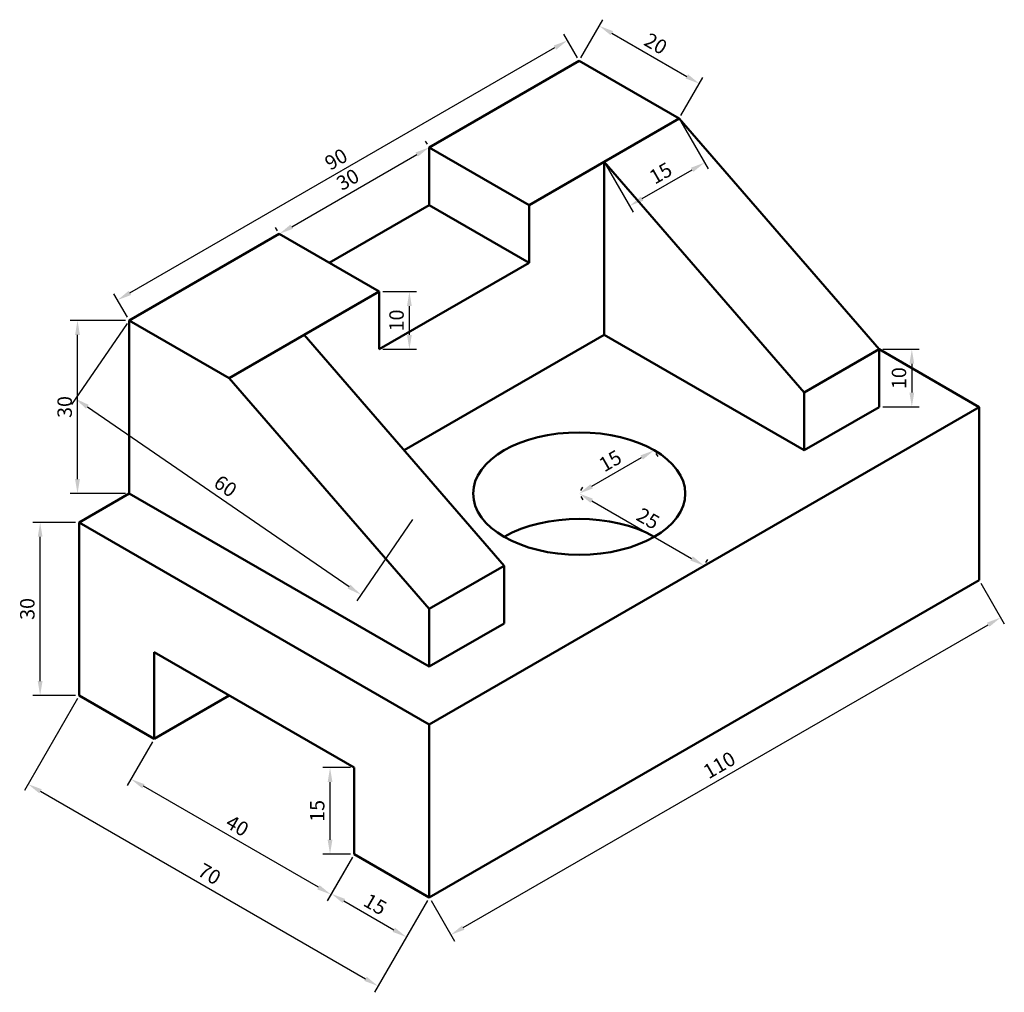
# Model space of a CAD drawing. Units: millimetres. Extents: x 2421 to 2592, y 893 to 1062.
import ezdxf

# ---------------------------------------------------------------- set-up
doc = ezdxf.new("R2010")
doc.units = ezdxf.units.MM
doc.layers.add('M-DIMS', color=2, linetype='Continuous', lineweight=25)
doc.layers.add('M-OUTL', color=7, linetype='Continuous', lineweight=50)
doc.styles.get("Standard").update_dxf_attribs({"font": 'arial.ttf'})
doc.dimstyles.new('ISO-25', dxfattribs={"dimtxt": 2.5, "dimasz": 2.5, "dimexe": 1.25, "dimexo": 0.625, "dimtad": 1, "dimtxsty": 'Standard', "dimcen": 2.5, "dimadec": 0, "dimazin": 0, "dimtfac": 1, "dimtmove": 0, "dimatfit": 3, "dimfxl": 1, "dimarcsym": 0})

# ---------------------------------------------------------------- blocks, each defined once
blk = doc.blocks.new('*D1')
at = {"layer": 'Defpoints', "color": 0, "transparency": 16777216}
for p in [(2424.82, 974.94), (2431.59, 974.94), (2431.59, 944.94)]:
    blk.add_point(p, dxfattribs=at)
at = {"layer": 'M-DIMS', "color": 0, "lineweight": -2, "transparency": 16777216}
for p, q in [((2430.97, 974.94), (2423.57, 974.94)), ((2424.82, 947.44), (2424.82, 972.44)), ((2430.97, 944.94), (2423.57, 944.94))]:
    blk.add_line(p, q, dxfattribs=at)
at = {"layer": 'M-DIMS', "color": 0, "transparency": 16777216}
for points in [[(2424.4, 972.44), (2425.23, 972.44), (2424.82, 974.94)], [(2424.4, 947.44), (2425.23, 947.44), (2424.82, 944.94)]]:
    blk.add_solid(points, dxfattribs=at)
at = {"layer": 'M-DIMS', "color": 0, "transparency": 16777216, "insert": (2422.92, 959.94), "char_height": 2.5, "attachment_point": 5, "rotation": 90}
blk.add_mtext('30', dxfattribs=at)
blk = doc.blocks.new('*D2')
at = {"layer": 'Defpoints', "color": 0, "transparency": 16777216}
for p in [(2431.29, 1009.94), (2440.25, 1009.94), (2440.25, 979.94)]:
    blk.add_point(p, dxfattribs=at)
at = {"layer": 'M-DIMS', "color": 0, "lineweight": -2, "transparency": 16777216}
for p, q in [((2439.63, 1009.94), (2430.04, 1009.94)), ((2431.29, 982.44), (2431.29, 1007.44)), ((2439.63, 979.94), (2430.04, 979.94))]:
    blk.add_line(p, q, dxfattribs=at)
at = {"layer": 'M-DIMS', "color": 0, "transparency": 16777216}
for points in [[(2430.87, 1007.44), (2431.71, 1007.44), (2431.29, 1009.94)], [(2430.87, 982.44), (2431.71, 982.44), (2431.29, 979.94)]]:
    blk.add_solid(points, dxfattribs=at)
at = {"layer": 'M-DIMS', "color": 0, "transparency": 16777216, "insert": (2429.39, 994.94), "char_height": 2.5, "attachment_point": 5, "rotation": 90}
blk.add_mtext('30', dxfattribs=at)
blk = doc.blocks.new('*D3')
at = {"layer": 'Defpoints', "color": 0, "transparency": 16777216}
for p in [(2440.25, 1009.94), (2489.7, 975.96), (2480.39, 962.4)]:
    blk.add_point(p, dxfattribs=at)
at = {"layer": 'M-DIMS', "color": 0, "lineweight": -2, "transparency": 16777216}
for p, q in [((2439.9, 1009.42), (2430.23, 995.35)), ((2433, 994.96), (2478.33, 963.81)), ((2489.35, 975.44), (2479.68, 961.37))]:
    blk.add_line(p, q, dxfattribs=at)
at = {"layer": 'M-DIMS', "color": 0, "transparency": 16777216}
for points in [[(2433.23, 995.31), (2432.76, 994.62), (2430.94, 996.38)], [(2478.56, 964.16), (2478.09, 963.47), (2480.39, 962.4)]]:
    blk.add_solid(points, dxfattribs=at)
at = {"layer": 'M-DIMS', "color": 0, "transparency": 16777216, "insert": (2456.74, 980.96), "char_height": 2.5, "attachment_point": 5, "rotation": 325.5033}
blk.add_mtext('60', dxfattribs=at)
blk = doc.blocks.new('*D4')
at = {"layer": 'Defpoints', "color": 0, "transparency": 16777216}
for p in [(2516.16, 1058.47), (2518.2, 1054.94), (2440.25, 1009.94)]:
    blk.add_point(p, dxfattribs=at)
at = {"layer": 'M-DIMS', "color": 0, "lineweight": -2, "transparency": 16777216}
for p, q in [((2517.88, 1055.48), (2515.54, 1059.55)), ((2440.38, 1014.72), (2514, 1057.22)), ((2439.94, 1010.48), (2437.59, 1014.55))]:
    blk.add_line(p, q, dxfattribs=at)
at = {"layer": 'M-DIMS', "color": 0, "transparency": 16777216}
for points in [[(2513.79, 1057.58), (2514.2, 1056.85), (2516.16, 1058.47)], [(2440.17, 1015.08), (2440.59, 1014.35), (2438.22, 1013.47)]]:
    blk.add_solid(points, dxfattribs=at)
at = {"layer": 'M-DIMS', "color": 0, "transparency": 16777216, "insert": (2476.24, 1037.61), "char_height": 2.5, "attachment_point": 5, "rotation": 30}
blk.add_mtext('90', dxfattribs=at)
blk = doc.blocks.new('*D5')
at = {"layer": 'Defpoints', "color": 0, "transparency": 16777216}
for p in [(2518.2, 1054.94), (2539.01, 1050.98), (2535.52, 1044.94)]:
    blk.add_point(p, dxfattribs=at)
at = {"layer": 'M-DIMS', "color": 0, "lineweight": -2, "transparency": 16777216}
for p, q in [((2518.51, 1055.48), (2522.31, 1062.06)), ((2523.85, 1059.73), (2536.84, 1052.23)), ((2535.83, 1045.48), (2539.63, 1052.06))]:
    blk.add_line(p, q, dxfattribs=at)
at = {"layer": 'M-DIMS', "color": 0, "transparency": 16777216}
for points in [[(2524.06, 1060.09), (2523.64, 1059.37), (2521.69, 1060.98)], [(2537.05, 1052.59), (2536.63, 1051.87), (2539.01, 1050.98)]]:
    blk.add_solid(points, dxfattribs=at)
at = {"layer": 'M-DIMS', "color": 0, "transparency": 16777216, "insert": (2531.3, 1057.63), "char_height": 2.5, "attachment_point": 5, "rotation": 330}
blk.add_mtext('20', dxfattribs=at)
blk = doc.blocks.new('*D6')
at = {"layer": 'Defpoints', "color": 0, "transparency": 16777216}
for p in [(2535.52, 1044.94), (2522.53, 1037.44), (2539.93, 1037.3)]:
    blk.add_point(p, dxfattribs=at)
at = {"layer": 'M-DIMS', "color": 0, "lineweight": -2, "transparency": 16777216}
for p, q in [((2535.83, 1044.4), (2540.55, 1036.21)), ((2522.84, 1036.9), (2527.56, 1028.71)), ((2529.1, 1031.05), (2537.76, 1036.05))]:
    blk.add_line(p, q, dxfattribs=at)
at = {"layer": 'M-DIMS', "color": 0, "transparency": 16777216}
for points in [[(2537.56, 1036.41), (2537.97, 1035.69), (2539.93, 1037.3)], [(2528.9, 1031.41), (2529.31, 1030.69), (2526.94, 1029.8)]]:
    blk.add_solid(points, dxfattribs=at)
at = {"layer": 'M-DIMS', "color": 0, "transparency": 16777216, "insert": (2532.48, 1035.19), "char_height": 2.5, "attachment_point": 5, "rotation": 30}
blk.add_mtext('15', dxfattribs=at)
blk = doc.blocks.new('*D7')
at = {"layer": 'Defpoints', "color": 0, "transparency": 16777216}
for p in [(2518.2, 979.94), (2539.85, 967.44), (2539.85, 967.44)]:
    blk.add_point(p, dxfattribs=at)
at = {"layer": 'M-DIMS', "color": 0, "lineweight": -2, "transparency": 16777216}
for p, q in [((2518.51, 980.48), (2518.82, 981.02)), ((2520.36, 978.69), (2537.68, 968.69)), ((2540.16, 967.98), (2540.47, 968.52))]:
    blk.add_line(p, q, dxfattribs=at)
at = {"layer": 'M-DIMS', "color": 0, "transparency": 16777216}
for points in [[(2520.57, 979.05), (2520.15, 978.33), (2518.2, 979.94)], [(2537.89, 969.05), (2537.47, 968.33), (2539.85, 967.44)]]:
    blk.add_solid(points, dxfattribs=at)
at = {"layer": 'M-DIMS', "color": 0, "transparency": 16777216, "insert": (2529.97, 975.33), "char_height": 2.5, "attachment_point": 5, "rotation": 330}
blk.add_mtext('25', dxfattribs=at)
blk = doc.blocks.new('*D8')
at = {"layer": 'Defpoints', "color": 0, "transparency": 16777216}
for p in [(2531.19, 987.44), (2531.19, 987.44), (2518.2, 979.94)]:
    blk.add_point(p, dxfattribs=at)
at = {"layer": 'M-DIMS', "color": 0, "lineweight": -2, "transparency": 16777216}
for p, q in [((2520.36, 981.19), (2529.02, 986.19)), ((2531.5, 986.9), (2531.81, 986.36)), ((2518.51, 979.4), (2518.82, 978.86))]:
    blk.add_line(p, q, dxfattribs=at)
at = {"layer": 'M-DIMS', "color": 0, "transparency": 16777216}
for points in [[(2528.81, 986.55), (2529.23, 985.83), (2531.19, 987.44)], [(2520.15, 981.55), (2520.57, 980.83), (2518.2, 979.94)]]:
    blk.add_solid(points, dxfattribs=at)
at = {"layer": 'M-DIMS', "color": 0, "transparency": 16777216, "insert": (2523.74, 985.33), "char_height": 2.5, "attachment_point": 5, "rotation": 30}
blk.add_mtext('15', dxfattribs=at)
blk = doc.blocks.new('*D9')
at = {"layer": 'Defpoints', "color": 0, "transparency": 16777216}
for p in [(2570.16, 1004.94), (2570.16, 994.94), (2575.82, 994.94)]:
    blk.add_point(p, dxfattribs=at)
at = {"layer": 'M-DIMS', "color": 0, "lineweight": -2, "transparency": 16777216}
for p, q in [((2570.78, 1004.94), (2577.07, 1004.94)), ((2575.82, 1002.44), (2575.82, 997.44)), ((2570.78, 994.94), (2577.07, 994.94))]:
    blk.add_line(p, q, dxfattribs=at)
at = {"layer": 'M-DIMS', "color": 0, "transparency": 16777216}
for points in [[(2575.41, 1002.44), (2576.24, 1002.44), (2575.82, 1004.94)], [(2575.41, 997.44), (2576.24, 997.44), (2575.82, 994.94)]]:
    blk.add_solid(points, dxfattribs=at)
at = {"layer": 'M-DIMS', "color": 0, "transparency": 16777216, "insert": (2573.92, 999.94), "char_height": 2.5, "attachment_point": 5, "rotation": 90}
blk.add_mtext('10', dxfattribs=at)
blk = doc.blocks.new('*D10')
at = {"layer": 'Defpoints', "color": 0, "transparency": 16777216}
for p in [(2483.56, 1014.94), (2488.78, 1014.94), (2483.56, 1004.94)]:
    blk.add_point(p, dxfattribs=at)
at = {"layer": 'M-DIMS', "color": 0, "lineweight": -2, "transparency": 16777216}
for p, q in [((2484.18, 1014.94), (2490.03, 1014.94)), ((2488.78, 1007.44), (2488.78, 1012.44)), ((2484.18, 1004.94), (2490.03, 1004.94))]:
    blk.add_line(p, q, dxfattribs=at)
at = {"layer": 'M-DIMS', "color": 0, "transparency": 16777216}
for points in [[(2488.37, 1012.44), (2489.2, 1012.44), (2488.78, 1014.94)], [(2488.37, 1007.44), (2489.2, 1007.44), (2488.78, 1004.94)]]:
    blk.add_solid(points, dxfattribs=at)
at = {"layer": 'M-DIMS', "color": 0, "transparency": 16777216, "insert": (2486.88, 1009.94), "char_height": 2.5, "attachment_point": 5, "rotation": 90}
blk.add_mtext('10', dxfattribs=at)
blk = doc.blocks.new('*D11')
at = {"layer": 'Defpoints', "color": 0, "transparency": 16777216}
for p in [(2475.04, 932.44), (2479.23, 932.44), (2479.23, 917.44)]:
    blk.add_point(p, dxfattribs=at)
at = {"layer": 'M-DIMS', "color": 0, "lineweight": -2, "transparency": 16777216}
for p, q in [((2478.6, 932.44), (2473.79, 932.44)), ((2475.04, 919.94), (2475.04, 929.94)), ((2478.6, 917.44), (2473.79, 917.44))]:
    blk.add_line(p, q, dxfattribs=at)
at = {"layer": 'M-DIMS', "color": 0, "transparency": 16777216}
for points in [[(2474.62, 929.94), (2475.45, 929.94), (2475.04, 932.44)], [(2474.62, 919.94), (2475.45, 919.94), (2475.04, 917.44)]]:
    blk.add_solid(points, dxfattribs=at)
at = {"layer": 'M-DIMS', "color": 0, "transparency": 16777216, "insert": (2473.14, 924.94), "char_height": 2.5, "attachment_point": 5, "rotation": 90}
blk.add_mtext('15', dxfattribs=at)
blk = doc.blocks.new('*D12')
at = {"layer": 'Defpoints', "color": 0, "transparency": 16777216}
for p in [(2587.48, 964.94), (2591.22, 958.46), (2492.22, 909.94)]:
    blk.add_point(p, dxfattribs=at)
at = {"layer": 'M-DIMS', "color": 0, "lineweight": -2, "transparency": 16777216}
for p, q in [((2587.79, 964.4), (2591.84, 957.38)), ((2498.12, 904.71), (2589.05, 957.21)), ((2492.53, 909.4), (2496.58, 902.38))]:
    blk.add_line(p, q, dxfattribs=at)
at = {"layer": 'M-DIMS', "color": 0, "transparency": 16777216}
for points in [[(2588.84, 957.57), (2589.26, 956.85), (2591.22, 958.46)], [(2497.91, 905.07), (2498.33, 904.35), (2495.95, 903.46)]]:
    blk.add_solid(points, dxfattribs=at)
at = {"layer": 'M-DIMS', "color": 0, "transparency": 16777216, "insert": (2542.63, 932.61), "char_height": 2.5, "attachment_point": 5, "rotation": 30}
blk.add_mtext('110', dxfattribs=at)
blk = doc.blocks.new('*D13')
at = {"layer": 'Defpoints', "color": 0, "transparency": 16777216}
for p in [(2444.58, 937.44), (2440.55, 930.45), (2479.23, 917.44)]:
    blk.add_point(p, dxfattribs=at)
at = {"layer": 'M-DIMS', "color": 0, "lineweight": -2, "transparency": 16777216}
for p, q in [((2444.27, 936.9), (2439.92, 929.36)), ((2473.02, 911.7), (2442.71, 929.2)), ((2478.91, 916.9), (2474.56, 909.36))]:
    blk.add_line(p, q, dxfattribs=at)
at = {"layer": 'M-DIMS', "color": 0, "transparency": 16777216}
for points in [[(2442.92, 929.56), (2442.51, 928.84), (2440.55, 930.45)], [(2473.23, 912.06), (2472.82, 911.34), (2475.19, 910.45)]]:
    blk.add_solid(points, dxfattribs=at)
at = {"layer": 'M-DIMS', "color": 0, "transparency": 16777216, "insert": (2458.82, 922.09), "char_height": 2.5, "attachment_point": 5, "rotation": 330}
blk.add_mtext('40', dxfattribs=at)
blk = doc.blocks.new('*D14')
at = {"layer": 'Defpoints', "color": 0, "transparency": 16777216}
for p in [(2431.59, 944.94), (2492.22, 909.94), (2483.35, 894.58)]:
    blk.add_point(p, dxfattribs=at)
at = {"layer": 'M-DIMS', "color": 0, "lineweight": -2, "transparency": 16777216}
for p, q in [((2431.28, 944.4), (2422.1, 928.5)), ((2424.89, 928.33), (2481.18, 895.83)), ((2491.9, 909.4), (2482.72, 893.5))]:
    blk.add_line(p, q, dxfattribs=at)
at = {"layer": 'M-DIMS', "color": 0, "transparency": 16777216}
for points in [[(2425.1, 928.69), (2424.68, 927.97), (2422.73, 929.58)], [(2481.39, 896.19), (2480.98, 895.47), (2483.35, 894.58)]]:
    blk.add_solid(points, dxfattribs=at)
at = {"layer": 'M-DIMS', "color": 0, "transparency": 16777216, "insert": (2453.99, 913.73), "char_height": 2.5, "attachment_point": 5, "rotation": 330}
blk.add_mtext('70', dxfattribs=at)
blk = doc.blocks.new('*D15')
at = {"layer": 'Defpoints', "color": 0, "transparency": 16777216}
for p in [(2479.23, 917.44), (2492.22, 909.94), (2488.26, 903.08)]:
    blk.add_point(p, dxfattribs=at)
at = {"layer": 'M-DIMS', "color": 0, "lineweight": -2, "transparency": 16777216}
for p, q in [((2478.91, 916.9), (2474.64, 909.5)), ((2477.43, 909.33), (2486.09, 904.33)), ((2491.9, 909.4), (2487.63, 902))]:
    blk.add_line(p, q, dxfattribs=at)
at = {"layer": 'M-DIMS', "color": 0, "transparency": 16777216}
for points in [[(2477.64, 909.69), (2477.22, 908.97), (2475.27, 910.58)], [(2486.3, 904.69), (2485.88, 903.97), (2488.26, 903.08)]]:
    blk.add_solid(points, dxfattribs=at)
at = {"layer": 'M-DIMS', "color": 0, "transparency": 16777216, "insert": (2482.71, 908.48), "char_height": 2.5, "attachment_point": 5, "rotation": 330}
blk.add_mtext('15', dxfattribs=at)
blk = doc.blocks.new('*D16')
at = {"layer": 'Defpoints', "color": 0, "transparency": 16777216}
for p in [(2492.22, 1039.94), (2492.22, 1039.94), (2466.24, 1024.94)]:
    blk.add_point(p, dxfattribs=at)
at = {"layer": 'M-DIMS', "color": 0, "lineweight": -2, "transparency": 16777216}
for p, q in [((2491.9, 1040.48), (2491.59, 1041.02)), ((2468.4, 1026.19), (2490.05, 1038.69)), ((2465.92, 1025.48), (2465.61, 1026.02))]:
    blk.add_line(p, q, dxfattribs=at)
at = {"layer": 'M-DIMS', "color": 0, "transparency": 16777216}
for points in [[(2489.84, 1039.05), (2490.26, 1038.33), (2492.22, 1039.94)], [(2468.19, 1026.55), (2468.61, 1025.83), (2466.24, 1024.94)]]:
    blk.add_solid(points, dxfattribs=at)
at = {"layer": 'M-DIMS', "color": 0, "transparency": 16777216, "insert": (2478.27, 1034.09), "char_height": 2.5, "attachment_point": 5, "rotation": 30}
blk.add_mtext('30', dxfattribs=at)

msp = doc.modelspace()

# ---------------------------------------------------------------- linework, layer by layer
at = {"layer": 'M-OUTL'}
for p, q in [((2492.216, 1039.938), (2518.197, 1054.938)), ((2518.197, 1054.938), (2535.517, 1044.938)), ((2535.517, 1044.938), (2509.536, 1029.938)), ((2535.517, 1044.938), (2570.158, 1004.938)), ((2509.536, 1029.938), (2492.216, 1039.938)), ((2492.216, 1029.938), (2492.216, 1039.938)), ((2522.527, 1007.438), (2522.527, 1037.438)), ((2522.527, 1037.438), (2557.168, 997.438)), ((2492.216, 1029.938), (2474.895, 1019.938)), ((2509.536, 1019.938), (2492.216, 1029.938)), ((2509.536, 1019.938), (2509.536, 1029.938)), ((2440.254, 1009.938), (2466.235, 1024.938)), ((2466.235, 1024.938), (2483.556, 1014.938)), ((2483.556, 1004.938), (2509.536, 1019.938)), ((2457.575, 999.938), (2483.556, 1014.938)), ((2483.556, 1014.938), (2483.556, 1004.938)), ((2440.254, 979.938), (2440.254, 1009.938)), ((2440.254, 1009.938), (2457.575, 999.938)), ((2470.565, 1007.438), (2505.206, 967.438)), ((2522.527, 1007.438), (2487.886, 987.438)), ((2557.168, 987.438), (2522.527, 1007.438)), ((2570.158, 1004.938), (2557.168, 997.438)), ((2570.158, 994.938), (2570.158, 1004.938)), ((2578.818, 999.938), (2570.158, 1004.938)), ((2457.575, 999.938), (2492.216, 959.938)), ((2587.479, 994.938), (2578.818, 999.938)), ((2557.168, 997.438), (2557.168, 987.438)), ((2587.479, 994.938), (2492.216, 939.938)), ((2557.168, 987.438), (2570.158, 994.938)), ((2587.479, 964.938), (2587.479, 994.938)), ((2431.594, 974.938), (2440.254, 979.938)), ((2440.254, 979.938), (2492.216, 949.938)), ((2431.594, 944.938), (2431.594, 974.938)), ((2431.594, 974.938), (2492.216, 939.938)), ((2505.206, 967.438), (2492.216, 959.938)), ((2505.206, 957.438), (2505.206, 967.438)), ((2492.216, 909.938), (2587.479, 964.938)), ((2492.216, 959.938), (2492.216, 949.938)), ((2492.216, 949.938), (2505.206, 957.438)), ((2479.225, 932.438), (2444.584, 952.438)), ((2444.584, 952.438), (2444.584, 937.438)), ((2444.584, 937.438), (2431.594, 944.938)), ((2444.584, 937.438), (2457.575, 944.938)), ((2492.216, 939.938), (2492.216, 909.938)), ((2479.225, 917.438), (2479.225, 932.438)), ((2492.216, 909.938), (2479.225, 917.438))]:
    msp.add_line(p, q, dxfattribs=at)
msp.add_ellipse((2518.197, 979.938), major_axis=(-18.371, 0), ratio=0.5773503, dxfattribs=at)
msp.add_ellipse((2518.197, 964.938), major_axis=(18.371, 0), ratio=0.5773503, start_param=0.7853982, end_param=2.3561945, dxfattribs=at)

# ---------------------------------------------------------------- dimensions: what is measured, and where the dimension line sits
at = {"layer": 'M-DIMS'}
for p1, p2, distance, picture, middle in [((2518.197, 1054.938), (2535.517, 1044.938), 6.979, '*D5', (2531.297, 1057.629)), ((2440.254, 1009.938), (2518.197, 1054.938), 4.073, '*D4', (2476.238, 1037.612)), ((2522.527, 1037.438), (2535.517, 1044.938), -8.824, '*D6', (2532.483, 1035.193)), ((2466.235, 1024.938), (2492.216, 1039.938), 0, '*D16', (2478.274, 1034.085)), ((2440.254, 1009.938), (2489.704, 975.956), -16.45, '*D3', (2456.739, 980.957)), ((2518.197, 979.938), (2531.187, 987.438), 0, '*D8', (2523.741, 985.335)), ((2518.197, 979.938), (2539.847, 967.438), 0, '*D7', (2529.973, 975.335)), ((2492.216, 909.938), (2587.479, 964.938), -7.477, '*D12', (2542.635, 932.61)), ((2431.594, 944.938), (2492.216, 909.938), -17.735, '*D14', (2453.988, 913.726)), ((2479.225, 917.438), (2444.584, 937.438), 8.072, '*D13', (2458.82, 922.094)), ((2479.225, 917.438), (2492.216, 909.938), -7.917, '*D15', (2482.713, 908.478))]:
    dim = msp.add_aligned_dim(p1=p1, p2=p2, distance=distance, dimstyle='ISO-25', override={"dimclrd": 0, "dimclre": 0, "dimclrt": 0}, dxfattribs=at)
    dim.commit()
    dim.dimension.update_dxf_attribs({"geometry": picture, "text_midpoint": middle})
for base, p1, p2, picture, middle in [((2488.785, 1014.938), (2483.556, 1004.938), (2483.556, 1014.938), '*D10', (2486.883, 1009.938)), ((2431.291, 1009.938), (2440.254, 979.938), (2440.254, 1009.938), '*D2', (2429.389, 994.938)), ((2575.822, 994.938), (2570.158, 1004.938), (2570.158, 994.938), '*D9', (2573.921, 999.938)), ((2424.818, 974.938), (2431.594, 944.938), (2431.594, 974.938), '*D1', (2422.916, 959.938)), ((2475.037, 932.438), (2479.225, 917.438), (2479.225, 932.438), '*D11', (2473.135, 924.938))]:
    dim = msp.add_linear_dim(base=base, p1=p1, p2=p2, angle=90, dimstyle='ISO-25', override={"dimclrd": 0, "dimclre": 0, "dimclrt": 0}, dxfattribs=at)
    dim.commit()
    dim.dimension.update_dxf_attribs({"geometry": picture, "text_midpoint": middle})

doc.saveas('drawing.dxf')
